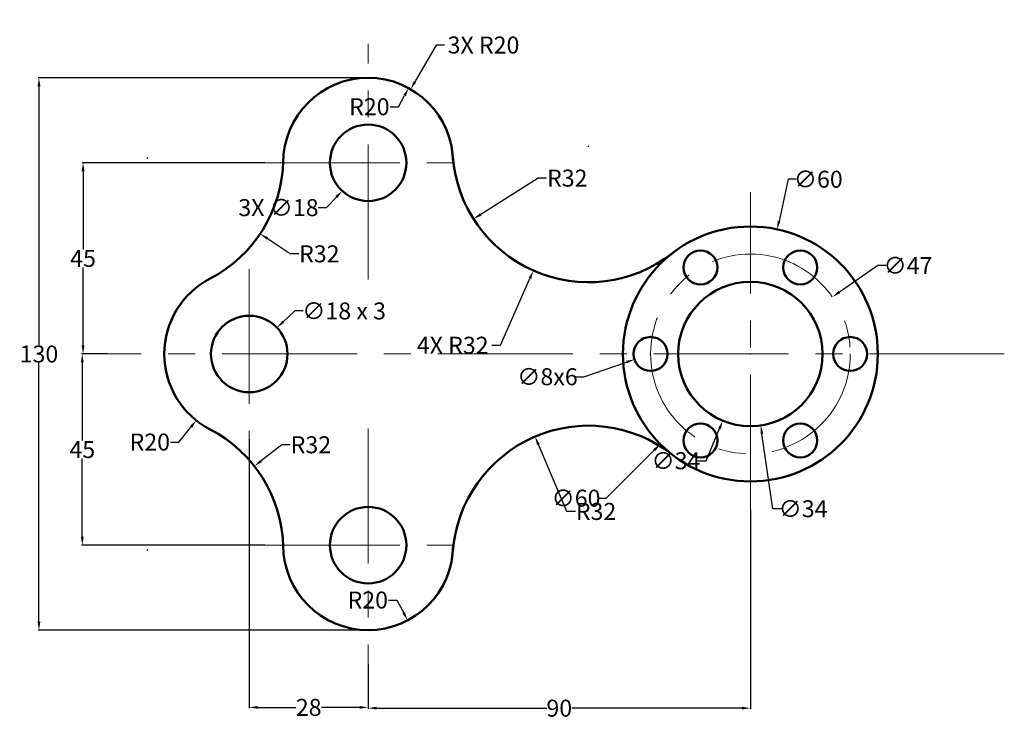
# Model space of a CAD drawing. Units: inches. Extents: x 313 to 545, y 238 to 402.
import ezdxf

# ---------------------------------------------------------------- set-up
doc = ezdxf.new("R2010")
doc.units = ezdxf.units.IN
doc.header["$MEASUREMENT"] = 0
doc.linetypes.add('CENTER', pattern=[50.8, 31.75, -6.35, 6.35, -6.35])
for name, color, linetype, lineweight in [('M-CNTR', 4, 'CENTER', 18), ('M-DIMS', 2, 'Continuous', 25), ('M-OUTL', 7, 'Continuous', 50)]:
    doc.layers.add(name, color=color, linetype=linetype, lineweight=lineweight)
doc.styles.get("Standard").update_dxf_attribs({"font": 'arial.ttf'})
doc.dimstyles.get("Standard").update_dxf_attribs({"dimtxt": 4, "dimasz": 2, "dimexe": 0.18, "dimexo": 0.0625, "dimgap": 0.09, "dimtad": 0, "dimtih": 1, "dimtoh": 1, "dimdec": 0, "dimzin": 0, "dimdsep": 46, "dimtxsty": 'Standard', "dimcen": 0.09, "dimadec": 0, "dimazin": 0, "dimtfac": 1, "dimtdec": 0, "dimtofl": 0, "dimtmove": 0, "dimatfit": 3, "dimfxl": 1, "dimtolj": 1, "dimtzin": 0, "dimarcsym": 0})

# ---------------------------------------------------------------- blocks, each defined once
blk = doc.blocks.new('*U1')
blk.add_circle((0, 0), 4)
blk = doc.blocks.new('*U2')
at = {"layer": 'M-OUTL', "color": 0, "linetype": 'ByBlock', "lineweight": -2, "transparency": 16777216}
for p, rotation in [((473.38, 343.96), 119.9999999999999), ((496.88, 343.96), 59.99999999999999), ((461.63, 323.6), 180), ((473.38, 303.25), 239.9999999999999), ((496.88, 303.25), 299.9999999999999)]:
    blk.add_blockref('*U1', p, dxfattribs=dict(at, rotation=rotation))
blk.add_blockref('*U1', (508.63, 323.6), dxfattribs=at)
blk = doc.blocks.new('*D3')
at = {"layer": 'Defpoints', "color": 0, "transparency": 16777216}
for p in [(370.84, 368.6), (328.01, 323.6), (333.78, 323.6)]:
    blk.add_point(p, dxfattribs=at)
at = {"layer": 'M-DIMS', "color": 0, "lineweight": -2, "transparency": 16777216}
for p, q in [((370.77, 368.6), (327.83, 368.6)), ((328.01, 366.6), (328.01, 348.23)), ((328.01, 325.6), (328.01, 343.98)), ((333.72, 323.6), (327.83, 323.6))]:
    blk.add_line(p, q, dxfattribs=at)
at = {"layer": 'M-DIMS', "color": 0, "transparency": 16777216}
for points in [[(327.67, 366.6), (328.34, 366.6), (328.01, 368.6)], [(327.67, 325.6), (328.34, 325.6), (328.01, 323.6)]]:
    blk.add_solid(points, dxfattribs=at)
at = {"layer": 'M-DIMS', "color": 0, "transparency": 16777216, "insert": (328.01, 346.1), "char_height": 4, "attachment_point": 5}
blk.add_mtext('\\A1;45', dxfattribs=at)
blk = doc.blocks.new('*D4')
at = {"layer": 'Defpoints', "color": 0, "transparency": 16777216}
for p in [(333.78, 323.6), (327.83, 278.6), (370.84, 278.6)]:
    blk.add_point(p, dxfattribs=at)
at = {"layer": 'M-DIMS', "color": 0, "lineweight": -2, "transparency": 16777216}
for p, q in [((333.72, 323.6), (327.65, 323.6)), ((327.83, 321.6), (327.83, 303.23)), ((327.83, 280.6), (327.83, 298.98)), ((370.77, 278.6), (327.65, 278.6))]:
    blk.add_line(p, q, dxfattribs=at)
at = {"layer": 'M-DIMS', "color": 0, "transparency": 16777216}
for points in [[(327.49, 321.6), (328.16, 321.6), (327.83, 323.6)], [(327.49, 280.6), (328.16, 280.6), (327.83, 278.6)]]:
    blk.add_solid(points, dxfattribs=at)
at = {"layer": 'M-DIMS', "color": 0, "transparency": 16777216, "insert": (327.83, 301.1), "char_height": 4, "attachment_point": 5}
blk.add_mtext('\\A1;45', dxfattribs=at)
blk = doc.blocks.new('*D5')
at = {"layer": 'Defpoints', "color": 0, "transparency": 16777216}
for p in [(434.42, 304.15), (446.99, 274.73)]:
    blk.add_point(p, dxfattribs=at)
at = {"layer": 'M-DIMS', "color": 0, "lineweight": -2, "transparency": 16777216}
for p, q in [((441.94, 286.54), (435.2, 302.31)), ((443.94, 286.54), (441.94, 286.54))]:
    blk.add_line(p, q, dxfattribs=at)
at = {"layer": 'M-DIMS', "color": 0, "transparency": 16777216}
blk.add_solid([(435.51, 302.45), (434.9, 302.18), (434.42, 304.15)], dxfattribs=at)
at = {"layer": 'M-DIMS', "color": 0, "transparency": 16777216, "insert": (448.79, 286.54), "char_height": 4, "attachment_point": 5}
blk.add_mtext('\\A1;R32', dxfattribs=at)
blk = doc.blocks.new('*D6')
at = {"layer": 'Defpoints', "color": 0, "transparency": 16777216}
for p in [(446.99, 372.48), (419.95, 355.37)]:
    blk.add_point(p, dxfattribs=at)
at = {"layer": 'M-DIMS', "color": 0, "lineweight": -2, "transparency": 16777216}
for p, q in [((435.16, 364.99), (421.64, 356.44)), ((437.16, 364.99), (435.16, 364.99))]:
    blk.add_line(p, q, dxfattribs=at)
at = {"layer": 'M-DIMS', "color": 0, "transparency": 16777216}
blk.add_solid([(421.46, 356.72), (421.82, 356.16), (419.95, 355.37)], dxfattribs=at)
at = {"layer": 'M-DIMS', "color": 0, "transparency": 16777216, "insert": (442.01, 364.99), "char_height": 4, "attachment_point": 5}
blk.add_mtext('\\A1;R32', dxfattribs=at)
blk = doc.blocks.new('*D7')
at = {"layer": 'Defpoints', "color": 0, "transparency": 16777216}
for p in [(404.66, 386.19), (395.13, 368.6)]:
    blk.add_point(p, dxfattribs=at)
at = {"layer": 'M-DIMS', "color": 0, "lineweight": -2, "transparency": 16777216}
for p, q in [((402.28, 381.8), (403.71, 384.43)), ((400.28, 381.8), (402.28, 381.8))]:
    blk.add_line(p, q, dxfattribs=at)
at = {"layer": 'M-DIMS', "color": 0, "transparency": 16777216}
blk.add_solid([(403.42, 384.59), (404, 384.27), (404.66, 386.19)], dxfattribs=at)
at = {"layer": 'M-DIMS', "color": 0, "transparency": 16777216, "insert": (395.42, 381.8), "char_height": 4, "attachment_point": 5}
blk.add_mtext('\\A1;R20', dxfattribs=at)
blk = doc.blocks.new('*D8')
at = {"layer": 'Defpoints', "color": 0, "transparency": 16777216}
for p in [(343.15, 369.74), (369.72, 351.91)]:
    blk.add_point(p, dxfattribs=at)
at = {"layer": 'M-DIMS', "color": 0, "lineweight": -2, "transparency": 16777216}
for p, q in [((343.06, 369.74), (343.24, 369.74)), ((343.15, 369.65), (343.15, 369.83)), ((376.78, 347.17), (371.38, 350.8)), ((378.78, 347.17), (376.78, 347.17))]:
    blk.add_line(p, q, dxfattribs=at)
at = {"layer": 'M-DIMS', "color": 0, "transparency": 16777216}
blk.add_solid([(371.57, 351.07), (371.19, 350.52), (369.72, 351.91)], dxfattribs=at)
at = {"layer": 'M-DIMS', "color": 0, "transparency": 16777216, "insert": (383.63, 347.17), "char_height": 4, "attachment_point": 5}
blk.add_mtext('\\A1;R32', dxfattribs=at)
blk = doc.blocks.new('*D9')
at = {"layer": 'Defpoints', "color": 0, "transparency": 16777216}
for p in [(368.35, 297.19), (343.15, 277.47)]:
    blk.add_point(p, dxfattribs=at)
at = {"layer": 'M-DIMS', "color": 0, "lineweight": -2, "transparency": 16777216}
for p, q in [((374.8, 302.23), (369.92, 298.42)), ((376.8, 302.23), (374.8, 302.23)), ((343.06, 277.47), (343.24, 277.47)), ((343.15, 277.38), (343.15, 277.56))]:
    blk.add_line(p, q, dxfattribs=at)
at = {"layer": 'M-DIMS', "color": 0, "transparency": 16777216}
blk.add_solid([(369.72, 298.68), (370.13, 298.16), (368.35, 297.19)], dxfattribs=at)
at = {"layer": 'M-DIMS', "color": 0, "transparency": 16777216, "insert": (381.65, 302.23), "char_height": 4, "attachment_point": 5}
blk.add_mtext('\\A1;R32', dxfattribs=at)
blk = doc.blocks.new('*D10')
at = {"layer": 'Defpoints', "color": 0, "transparency": 16777216}
for p in [(373.67, 329.79), (360.6, 317.42)]:
    blk.add_point(p, dxfattribs=at)
at = {"layer": 'M-DIMS', "color": 0, "lineweight": -2, "transparency": 16777216}
for p, q in [((377.84, 333.73), (375.13, 331.16)), ((379.84, 333.73), (377.84, 333.73)), ((367.04, 323.6), (367.22, 323.6)), ((367.13, 323.51), (367.13, 323.69))]:
    blk.add_line(p, q, dxfattribs=at)
at = {"layer": 'M-DIMS', "color": 0, "transparency": 16777216}
blk.add_solid([(374.9, 331.4), (375.36, 330.92), (373.67, 329.79)], dxfattribs=at)
at = {"layer": 'M-DIMS', "color": 0, "transparency": 16777216, "insert": (389.47, 333.73), "char_height": 4, "attachment_point": 5}
blk.add_mtext('\\A1;∅18 x 3', dxfattribs=at)
blk = doc.blocks.new('*D11')
at = {"layer": 'Defpoints', "color": 0, "transparency": 16777216}
for p in [(367.13, 323.6), (354.66, 307.97)]:
    blk.add_point(p, dxfattribs=at)
at = {"layer": 'M-DIMS', "color": 0, "lineweight": -2, "transparency": 16777216}
for p, q in [((367.04, 323.6), (367.22, 323.6)), ((367.13, 323.51), (367.13, 323.69)), ((350.58, 302.87), (353.41, 306.41)), ((348.58, 302.87), (350.58, 302.87))]:
    blk.add_line(p, q, dxfattribs=at)
at = {"layer": 'M-DIMS', "color": 0, "transparency": 16777216}
blk.add_solid([(353.15, 306.62), (353.67, 306.2), (354.66, 307.97)], dxfattribs=at)
at = {"layer": 'M-DIMS', "color": 0, "transparency": 16777216, "insert": (343.72, 302.87), "char_height": 4, "attachment_point": 5}
blk.add_mtext('\\A1;R20', dxfattribs=at)
blk = doc.blocks.new('*D12')
at = {"layer": 'Defpoints', "color": 0, "transparency": 16777216}
for p in [(395.13, 278.6), (404.43, 260.89)]:
    blk.add_point(p, dxfattribs=at)
at = {"layer": 'M-DIMS', "color": 0, "lineweight": -2, "transparency": 16777216}
for p, q in [((399.91, 265.69), (401.91, 265.69)), ((401.91, 265.69), (403.5, 262.66))]:
    blk.add_line(p, q, dxfattribs=at)
at = {"layer": 'M-DIMS', "color": 0, "transparency": 16777216}
blk.add_solid([(403.79, 262.82), (403.2, 262.51), (404.43, 260.89)], dxfattribs=at)
at = {"layer": 'M-DIMS', "color": 0, "transparency": 16777216, "insert": (395.04, 265.69), "char_height": 4, "attachment_point": 5}
blk.add_mtext('\\A1;R20', dxfattribs=at)
blk = doc.blocks.new('*D13')
at = {"layer": 'Defpoints', "color": 0, "transparency": 16777216}
for p in [(367.13, 303.6), (395.13, 250.63), (395.13, 240.42)]:
    blk.add_point(p, dxfattribs=at)
at = {"layer": 'M-DIMS', "color": 0, "lineweight": -2, "transparency": 16777216}
for p, q in [((367.13, 303.54), (367.13, 240.24)), ((395.13, 250.57), (395.13, 240.24)), ((369.13, 240.42), (378.14, 240.42)), ((393.13, 240.42), (384.13, 240.42))]:
    blk.add_line(p, q, dxfattribs=at)
at = {"layer": 'M-DIMS', "color": 0, "transparency": 16777216}
for points in [[(369.13, 240.75), (369.13, 240.09), (367.13, 240.42)], [(393.13, 240.75), (393.13, 240.09), (395.13, 240.42)]]:
    blk.add_solid(points, dxfattribs=at)
at = {"layer": 'M-DIMS', "color": 0, "transparency": 16777216, "insert": (381.13, 240.42), "char_height": 4, "attachment_point": 5}
blk.add_mtext('\\A1;28', dxfattribs=at)
blk = doc.blocks.new('*D14')
at = {"layer": 'Defpoints', "color": 0, "transparency": 16777216}
for p in [(485.13, 287), (395.13, 250.63), (485.13, 240.24)]:
    blk.add_point(p, dxfattribs=at)
at = {"layer": 'M-DIMS', "color": 0, "lineweight": -2, "transparency": 16777216}
for p, q in [((485.13, 286.93), (485.13, 240.06)), ((395.13, 250.57), (395.13, 240.06)), ((397.13, 240.24), (437.19, 240.24)), ((483.13, 240.24), (443.08, 240.24))]:
    blk.add_line(p, q, dxfattribs=at)
at = {"layer": 'M-DIMS', "color": 0, "transparency": 16777216}
for points in [[(397.13, 240.57), (397.13, 239.91), (395.13, 240.24)], [(483.13, 240.57), (483.13, 239.91), (485.13, 240.24)]]:
    blk.add_solid(points, dxfattribs=at)
at = {"layer": 'M-DIMS', "color": 0, "transparency": 16777216, "insert": (440.13, 240.24), "char_height": 4, "attachment_point": 5}
blk.add_mtext('\\A1;90', dxfattribs=at)
blk = doc.blocks.new('*D15')
at = {"layer": 'Defpoints', "color": 0, "transparency": 16777216}
for p in [(482.69, 340.43), (487.58, 306.78)]:
    blk.add_point(p, dxfattribs=at)
at = {"layer": 'M-DIMS', "color": 0, "lineweight": -2, "transparency": 16777216}
for p, q in [((485.04, 323.6), (485.22, 323.6)), ((485.13, 323.51), (485.13, 323.69)), ((490.42, 287.17), (487.86, 304.8)), ((492.42, 287.17), (490.42, 287.17))]:
    blk.add_line(p, q, dxfattribs=at)
at = {"layer": 'M-DIMS', "color": 0, "transparency": 16777216}
blk.add_solid([(488.19, 304.85), (487.53, 304.75), (487.58, 306.78)], dxfattribs=at)
at = {"layer": 'M-DIMS', "color": 0, "transparency": 16777216, "insert": (497.54, 287.17), "char_height": 4, "attachment_point": 5}
blk.add_mtext('\\A1;∅34', dxfattribs=at)
blk = doc.blocks.new('*D16')
at = {"layer": 'Defpoints', "color": 0, "transparency": 16777216}
for p in [(465.42, 324.89), (457.85, 322.32)]:
    blk.add_point(p, dxfattribs=at)
at = {"layer": 'M-DIMS', "color": 0, "lineweight": -2, "transparency": 16777216}
for p, q in [((461.54, 323.6), (461.72, 323.6)), ((461.63, 323.51), (461.63, 323.69)), ((445.88, 318.25), (455.95, 321.67)), ((443.88, 318.25), (445.88, 318.25))]:
    blk.add_line(p, q, dxfattribs=at)
at = {"layer": 'M-DIMS', "color": 0, "transparency": 16777216}
blk.add_solid([(455.85, 321.99), (456.06, 321.36), (457.85, 322.32)], dxfattribs=at)
at = {"layer": 'M-DIMS', "color": 0, "transparency": 16777216, "insert": (437.35, 318.25), "char_height": 4, "attachment_point": 5}
blk.add_mtext('\\A1;∅8x6', dxfattribs=at)
blk = doc.blocks.new('*D17')
at = {"layer": 'Defpoints', "color": 0, "transparency": 16777216}
for p in [(491.45, 352.93), (478.82, 294.28)]:
    blk.add_point(p, dxfattribs=at)
at = {"layer": 'M-DIMS', "color": 0, "lineweight": -2, "transparency": 16777216}
for p, q in [((493.99, 364.73), (491.87, 354.89)), ((495.99, 364.73), (493.99, 364.73)), ((485.04, 323.6), (485.22, 323.6)), ((485.13, 323.51), (485.13, 323.69))]:
    blk.add_line(p, q, dxfattribs=at)
at = {"layer": 'M-DIMS', "color": 0, "transparency": 16777216}
blk.add_solid([(491.54, 354.96), (492.19, 354.82), (491.45, 352.93)], dxfattribs=at)
at = {"layer": 'M-DIMS', "color": 0, "transparency": 16777216, "insert": (501.11, 364.73), "char_height": 4, "attachment_point": 5}
blk.add_mtext('\\A1;∅60', dxfattribs=at)
blk = doc.blocks.new('*D18')
at = {"layer": 'Defpoints', "color": 0, "transparency": 16777216}
for p in [(504.44, 337.01), (465.83, 310.2)]:
    blk.add_point(p, dxfattribs=at)
at = {"layer": 'M-DIMS', "color": 0, "lineweight": -2, "transparency": 16777216}
for p, q in [((515.1, 344.42), (506.08, 338.15)), ((517.1, 344.42), (515.1, 344.42)), ((485.04, 323.6), (485.22, 323.6)), ((485.13, 323.51), (485.13, 323.69))]:
    blk.add_line(p, q, dxfattribs=at)
at = {"layer": 'M-DIMS', "color": 0, "transparency": 16777216}
blk.add_solid([(505.89, 338.42), (506.27, 337.88), (504.44, 337.01)], dxfattribs=at)
at = {"layer": 'M-DIMS', "color": 0, "transparency": 16777216, "insert": (522.23, 344.42), "char_height": 4, "attachment_point": 5}
blk.add_mtext('\\A1;∅47', dxfattribs=at)
blk = doc.blocks.new('MOUNT-HOLE-D18')
blk.add_circle((9, 9), 9)
blk = doc.blocks.new('*D20')
at = {"layer": 'Defpoints', "color": 0, "transparency": 16777216}
for p in [(317.63, 388.6), (395.13, 388.6), (395.13, 258.6)]:
    blk.add_point(p, dxfattribs=at)
at = {"layer": 'M-DIMS', "color": 0, "lineweight": -2, "transparency": 16777216}
for p, q in [((395.07, 388.6), (317.45, 388.6)), ((317.63, 386.6), (317.63, 325.74)), ((317.63, 260.6), (317.63, 321.47)), ((395.07, 258.6), (317.45, 258.6))]:
    blk.add_line(p, q, dxfattribs=at)
at = {"layer": 'M-DIMS', "color": 0, "transparency": 16777216}
for points in [[(317.3, 386.6), (317.97, 386.6), (317.63, 388.6)], [(317.3, 260.6), (317.97, 260.6), (317.63, 258.6)]]:
    blk.add_solid(points, dxfattribs=at)
at = {"layer": 'M-DIMS', "color": 0, "transparency": 16777216, "insert": (317.63, 323.6), "char_height": 4, "attachment_point": 5}
blk.add_mtext('\\A1;130', dxfattribs=at)
blk = doc.blocks.new('*D21')
at = {"layer": 'Defpoints', "color": 0, "transparency": 16777216}
for p in [(405.13, 385.92), (395.13, 368.6)]:
    blk.add_point(p, dxfattribs=at)
at = {"layer": 'M-DIMS', "color": 0, "lineweight": -2, "transparency": 16777216}
for p, q in [((411.13, 396.32), (406.13, 387.66)), ((413.13, 396.32), (411.13, 396.32)), ((395.04, 368.6), (395.22, 368.6)), ((395.13, 368.51), (395.13, 368.69))]:
    blk.add_line(p, q, dxfattribs=at)
at = {"layer": 'M-DIMS', "color": 0, "transparency": 16777216}
blk.add_solid([(405.85, 387.82), (406.42, 387.49), (405.13, 385.92)], dxfattribs=at)
at = {"layer": 'M-DIMS', "color": 0, "transparency": 16777216, "insert": (422.29, 396.32), "char_height": 4, "attachment_point": 5}
blk.add_mtext('\\A1;3X R20', dxfattribs=at)
blk = doc.blocks.new('*D22')
at = {"layer": 'Defpoints', "color": 0, "transparency": 16777216}
for p in [(401.26, 375.2), (389.01, 362.01)]:
    blk.add_point(p, dxfattribs=at)
at = {"layer": 'M-DIMS', "color": 0, "lineweight": -2, "transparency": 16777216}
for p, q in [((395.04, 368.6), (395.22, 368.6)), ((395.13, 368.51), (395.13, 368.69)), ((385.34, 358.05), (387.65, 360.54)), ((383.34, 358.05), (385.34, 358.05))]:
    blk.add_line(p, q, dxfattribs=at)
at = {"layer": 'M-DIMS', "color": 0, "transparency": 16777216}
blk.add_solid([(387.41, 360.77), (387.9, 360.31), (389.01, 362.01)], dxfattribs=at)
at = {"layer": 'M-DIMS', "color": 0, "transparency": 16777216, "insert": (374.02, 358.05), "char_height": 4, "attachment_point": 5}
blk.add_mtext('\\A1;3X ∅18', dxfattribs=at)
blk = doc.blocks.new('*D23')
at = {"layer": 'Defpoints', "color": 0, "transparency": 16777216}
for p in [(446.99, 372.48), (434.04, 343.22)]:
    blk.add_point(p, dxfattribs=at)
at = {"layer": 'M-DIMS', "color": 0, "lineweight": -2, "transparency": 16777216}
for p, q in [((446.9, 372.48), (447.08, 372.48)), ((446.99, 372.39), (446.99, 372.57)), ((426.27, 325.66), (433.23, 341.39)), ((424.27, 325.66), (426.27, 325.66))]:
    blk.add_line(p, q, dxfattribs=at)
at = {"layer": 'M-DIMS', "color": 0, "transparency": 16777216}
blk.add_solid([(432.93, 341.52), (433.53, 341.25), (434.04, 343.22)], dxfattribs=at)
at = {"layer": 'M-DIMS', "color": 0, "transparency": 16777216, "insert": (415.04, 325.66), "char_height": 4, "attachment_point": 5}
blk.add_mtext('\\A1;4X R32', dxfattribs=at)
blk = doc.blocks.new('*D24')
at = {"layer": 'Defpoints', "color": 0, "transparency": 16777216}
for p in [(506.35, 344.82), (463.92, 302.39)]:
    blk.add_point(p, dxfattribs=at)
at = {"layer": 'M-DIMS', "color": 0, "lineweight": -2, "transparency": 16777216}
for p, q in [((485.04, 323.6), (485.22, 323.6)), ((485.13, 323.51), (485.13, 323.69)), ((451.19, 289.66), (462.51, 300.98)), ((449.19, 289.66), (451.19, 289.66))]:
    blk.add_line(p, q, dxfattribs=at)
at = {"layer": 'M-DIMS', "color": 0, "transparency": 16777216}
blk.add_solid([(462.27, 301.21), (462.74, 300.74), (463.92, 302.39)], dxfattribs=at)
at = {"layer": 'M-DIMS', "color": 0, "transparency": 16777216, "insert": (444.07, 289.66), "char_height": 4, "attachment_point": 5}
blk.add_mtext('\\A1;∅60', dxfattribs=at)
blk = doc.blocks.new('*D25')
at = {"layer": 'Defpoints', "color": 0, "transparency": 16777216}
for p in [(491.64, 339.31), (478.63, 307.9)]:
    blk.add_point(p, dxfattribs=at)
at = {"layer": 'M-DIMS', "color": 0, "lineweight": -2, "transparency": 16777216}
for p, q in [((485.04, 323.6), (485.22, 323.6)), ((485.13, 323.51), (485.13, 323.69)), ((474.73, 298.47), (477.87, 306.05)), ((472.73, 298.47), (474.73, 298.47))]:
    blk.add_line(p, q, dxfattribs=at)
at = {"layer": 'M-DIMS', "color": 0, "transparency": 16777216}
blk.add_solid([(477.56, 306.18), (478.17, 305.92), (478.63, 307.9)], dxfattribs=at)
at = {"layer": 'M-DIMS', "color": 0, "transparency": 16777216, "insert": (467.61, 298.47), "char_height": 4, "attachment_point": 5}
blk.add_mtext('\\A1;∅34', dxfattribs=at)

msp = doc.modelspace()

# ---------------------------------------------------------------- linework, layer by layer
at = {"layer": 'M-CNTR'}
for p, q in [((395.13, 341.16), (395.13, 396.58)), ((370.84, 368.6), (420.11, 368.6)), ((485.13, 287), (485.13, 361.66)), ((367.13, 343.6), (367.13, 303.6)), ((544.91, 323.6), (333.78, 323.6)), ((395.13, 306.05), (395.13, 250.63)), ((370.84, 278.6), (420.11, 278.6))]:
    msp.add_line(p, q, dxfattribs=at)
msp.add_circle((485.13, 323.6), 23.5, dxfattribs=at)
at = {"layer": 'M-OUTL'}
for radius in [30, 17]:
    msp.add_circle((485.13, 323.6), radius, dxfattribs=at)
for centre, radius, start, end in [((395.13, 368.6), 20, 0, 180), ((343.15, 369.74), 32, 297.471, 358.7474), ((446.99, 372.48), 32, 184.276, 307.9692), ((367.13, 323.6), 20, 117.471, 242.529), ((446.99, 274.73), 32, 52.0308, 175.724), ((343.15, 277.47), 32, 1.2526, 62.529), ((395.13, 278.6), 20, 180, 0)]:
    msp.add_arc(centre, radius, start, end, dxfattribs=at)

# ---------------------------------------------------------------- block references
for name, p in [('MOUNT-HOLE-D18', (386.13, 359.6)), ('*U2', (0, 0)), ('MOUNT-HOLE-D18', (358.13, 314.6)), ('MOUNT-HOLE-D18', (386.13, 269.6))]:
    msp.add_blockref(name, p, dxfattribs=at)

# ---------------------------------------------------------------- dimensions: what is measured, and where the dimension line sits
at = {"layer": 'M-DIMS'}
for center, mpoint, text, picture, middle in [((395.13, 368.6), (405.13, 385.92), '3X <>', '*D21', (422.29, 396.32)), ((446.99, 372.48), (434.04, 343.22), '4X <>', '*D23', (415.04, 325.66))]:
    dim = msp.add_radius_dim(center=center, mpoint=mpoint, text=text, dimstyle='Standard', override={"dimdec": 0, "dimlfac": 1, "dimrnd": 0, "dimzin": 0, "dimdsep": 46, "dimlunit": 2}, dxfattribs=at)
    dim.commit()
    dim.dimension.update_dxf_attribs({"geometry": picture, "text_midpoint": middle, "dimtype": 164})
for base, p1, p2, override, picture, middle in [((317.63, 388.6), (395.13, 258.6), (395.13, 388.6), {"dimdec": 0, "dimlfac": 1, "dimrnd": 0, "dimzin": 0, "dimdsep": 46, "dimlunit": 2}, '*D20', (317.63, 323.6)), ((328.01, 323.6), (370.84, 368.6), (333.78, 323.6), {"dimclrd": 0, "dimclre": 0, "dimclrt": 0}, '*D3', (328.01, 346.1)), ((327.83, 278.6), (333.78, 323.6), (370.84, 278.6), {"dimclrd": 0, "dimclre": 0, "dimclrt": 0}, '*D4', (327.83, 301.1))]:
    dim = msp.add_linear_dim(base=base, p1=p1, p2=p2, angle=90, dimstyle='Standard', override=override, dxfattribs=at)
    dim.commit()
    dim.dimension.update_dxf_attribs({"geometry": picture, "text_midpoint": middle})
for center, mpoint, picture, middle in [((395.13, 368.6), (404.66, 386.19), '*D7', (395.42, 381.8)), ((446.99, 372.48), (419.95, 355.37), '*D6', (442.01, 364.99)), ((343.15, 369.74), (369.72, 351.91), '*D8', (383.63, 347.17)), ((367.13, 323.6), (354.66, 307.97), '*D11', (343.72, 302.87)), ((343.15, 277.47), (368.35, 297.19), '*D9', (381.65, 302.23)), ((446.99, 274.73), (434.42, 304.15), '*D5', (448.79, 286.54)), ((395.13, 278.6), (404.43, 260.89), '*D12', (395.04, 265.69))]:
    dim = msp.add_radius_dim(center=center, mpoint=mpoint, dimstyle='Standard', override={"dimclrd": 0, "dimclre": 0, "dimclrt": 0}, dxfattribs=at)
    dim.commit()
    dim.dimension.update_dxf_attribs({"geometry": picture, "text_midpoint": middle, "dimtype": 164})
for p1, p2, text, override, picture, middle in [((401.26, 375.2), (389.01, 362.01), '3X <>', {"dimdec": 0, "dimlfac": 1, "dimrnd": 0, "dimzin": 0, "dimdsep": 46, "dimlunit": 2}, '*D22', (374.02, 358.05)), ((360.6, 317.42), (373.67, 329.79), '<> x 3', {"dimclrd": 0, "dimclre": 0, "dimclrt": 0}, '*D10', (389.47, 333.73)), ((465.42, 324.89), (457.85, 322.32), '<>x6', {"dimclrd": 0, "dimclre": 0, "dimclrt": 0}, '*D16', (437.35, 318.25))]:
    dim = msp.add_diameter_dim_2p(p1=p1, p2=p2, text=text, dimstyle='Standard', override=override, dxfattribs=at)
    dim.commit()
    dim.dimension.update_dxf_attribs({"geometry": picture, "text_midpoint": middle, "dimtype": 163})
for p1, p2, override, picture, middle in [((478.82, 294.28), (491.45, 352.93), {"dimclrd": 0, "dimclre": 0, "dimclrt": 0}, '*D17', (501.11, 364.73)), ((465.83, 310.2), (504.44, 337.01), {"dimclrd": 0, "dimclre": 0, "dimclrt": 0}, '*D18', (522.23, 344.42)), ((506.35, 344.82), (463.92, 302.39), {"dimdec": 0, "dimlfac": 1, "dimrnd": 0, "dimzin": 0, "dimdsep": 46, "dimlunit": 2}, '*D24', (444.07, 289.66)), ((491.64, 339.31), (478.63, 307.9), {"dimdec": 0, "dimlfac": 1, "dimrnd": 0, "dimzin": 0, "dimdsep": 46, "dimlunit": 2}, '*D25', (467.61, 298.47)), ((482.69, 340.43), (487.58, 306.78), {"dimclrd": 0, "dimclre": 0, "dimclrt": 0}, '*D15', (497.54, 287.17))]:
    dim = msp.add_diameter_dim_2p(p1=p1, p2=p2, dimstyle='Standard', override=override, dxfattribs=at)
    dim.commit()
    dim.dimension.update_dxf_attribs({"geometry": picture, "text_midpoint": middle, "dimtype": 163})
for base, p1, p2, picture, middle in [((395.13, 240.42), (367.13, 303.6), (395.13, 250.63), '*D13', (381.13, 240.42)), ((485.13, 240.24), (395.13, 250.63), (485.13, 287), '*D14', (440.13, 240.24))]:
    dim = msp.add_linear_dim(base=base, p1=p1, p2=p2, dimstyle='Standard', override={"dimclrd": 0, "dimclre": 0, "dimclrt": 0}, dxfattribs=at)
    dim.commit()
    dim.dimension.update_dxf_attribs({"geometry": picture, "text_midpoint": middle})

doc.saveas('drawing.dxf')
